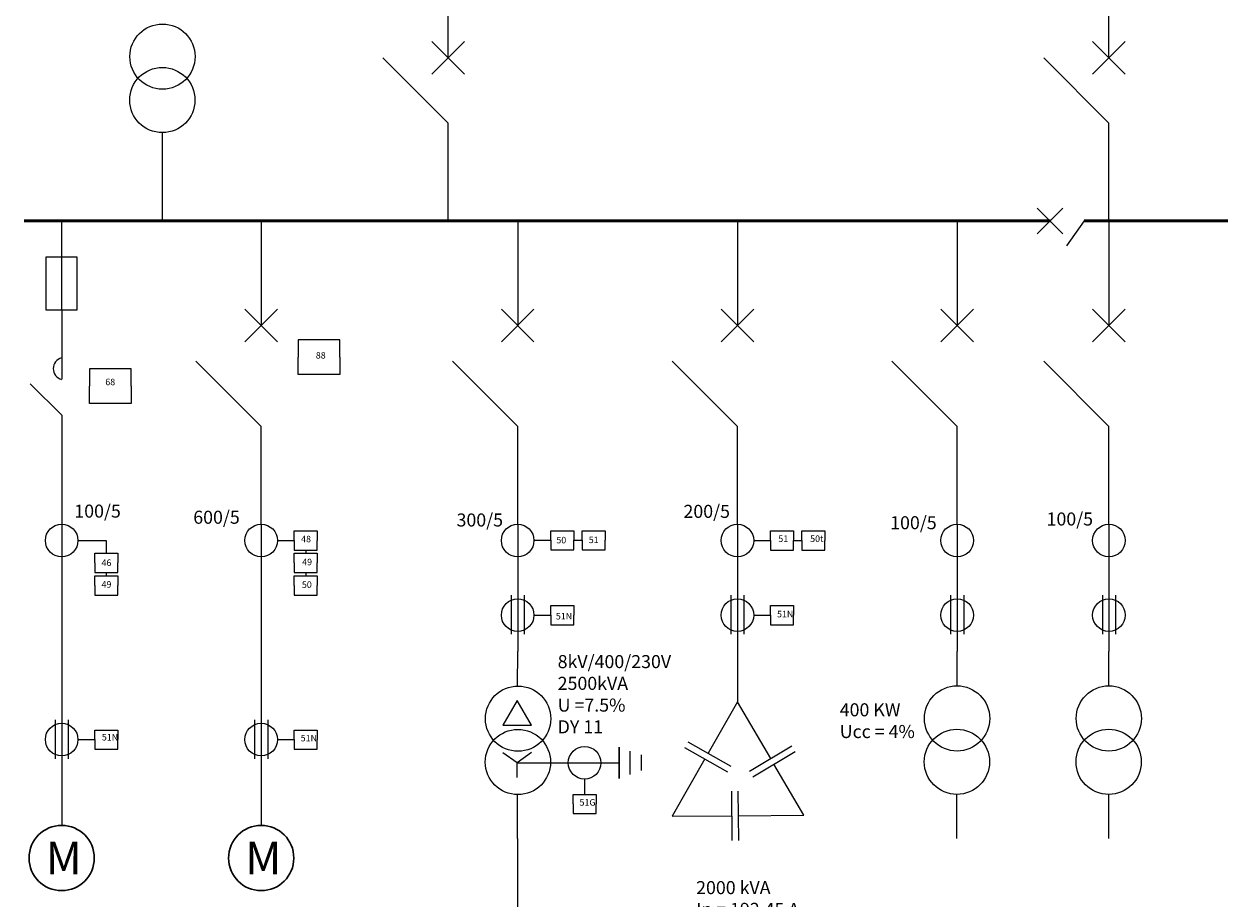
# Model space of a CAD drawing. Units: inches. Extents: x 77.1 to 95.7, y 45.4 to 81.6.
# Tile 2 of 3: x 77.2 to 95.6, y 58.2 to 71.6. Entities that reach past the tile are written whole.
import ezdxf

# ---------------------------------------------------------------- set-up
doc = ezdxf.new("R2010")
doc.units = ezdxf.units.IN
doc.header["$MEASUREMENT"] = 0
for name, color, linetype, lineweight in [('E-ANNO-TEXT', 7, 'Continuous', 18), ('E-POWR-BUSB', 7, 'Continuous', 50), ('E-POWR-CAPB', 3, 'Continuous', 25), ('E-POWR-CT', 4, 'Continuous', 18), ('E-POWR-EQPM', 3, 'Continuous', 30), ('E-POWR-FEED', 7, 'Continuous', 25), ('E-POWR-GRND', 3, 'Continuous', 18), ('E-POWR-SWCH', 1, 'Continuous', 25), ('E-POWR-XFMR', 4, 'Continuous', 25), ('E-PROT-RELY', 2, 'Continuous', 18), ('E-PROT-TEXT', 7, 'Continuous', 13), ('E-PROT-WIRE', 5, 'Continuous', 13)]:
    doc.layers.add(name, color=color, linetype=linetype, lineweight=lineweight)
doc.styles.get("Standard").update_dxf_attribs({"font": 'arial.ttf'})

# ---------------------------------------------------------------- blocks, each defined once
blk = doc.blocks.new('XFMR-TWO-WINDING')
for centre in [(0.502, 1.166), (0.5, 0.5)]:
    blk.add_circle(centre, 0.5)
blk = doc.blocks.new('CT-RESIDUAL')
for p, q in [((0.15, 0.598), (0.15, 0)), ((0.35, 0.598), (0.35, 0))]:
    blk.add_line(p, q)
blk.add_circle((0.25, 0.294), 0.25)
blk = doc.blocks.new('CT-SINGLE')
blk.add_circle((0.25, 0.25), 0.25)
blk = doc.blocks.new('MOTOR-AC')
blk.add_circle((0.5, 0.5), 0.5)
at = {"insert": (0.255, 0.75), "char_height": 0.5, "attachment_point": 1}
blk.add_mtext_dynamic_manual_height_columns('M', width=0.27964, gutter_width=1, heights=[0], dxfattribs=at)
blk = doc.blocks.new('EARTH-GROUND')
for p, q in [((0.174, 0.421), (0.174, 0.059)), ((0, 0.36), (0, 0.12))]:
    blk.add_line(p, q)
for points in [[(0.342, 0.24), (0.342, 0.24), (0.342, 0.48), (0.342, 0.48)], [(0.342, 0.24), (0.342, 0.24), (0.342, 0), (0.342, 0)]]:
    blk.add_lwpolyline(points, close=True)
blk = doc.blocks.new('CB-INCOMER-OPEN')
for p, q in [((0.75, 0.75), (1.25, 1.25)), ((0.75, 1.25), (1.25, 0.75)), ((1, 0), (0, 1))]:
    blk.add_line(p, q)
blk = doc.blocks.new('CB-FEEDER-OPEN')
for p, q in [((0.75, 1.299), (1.25, 1.799)), ((0.75, 1.799), (1.25, 1.299)), ((1, 0), (0, 1))]:
    blk.add_line(p, q)
blk = doc.blocks.new('RELAY-FUNCTION')
for p, q in [((0, 0.148), (0, 0.295)), ((0, 0.295), (0.353, 0.295)), ((0.353, 0.295), (0.353, 0.148)), ((0, 0.148), (0, 0)), ((0, 0), (0.353, 0)), ((0.353, 0), (0.353, 0.148))]:
    blk.add_line(p, q)
blk = doc.blocks.new('RELAY-FUNCTION-MED')
for p, q in [((0.638, 0.533), (0, 0.533)), ((0, 0.533), (0, 0.266)), ((0.638, 0.266), (0.638, 0.533)), ((0, 0), (0, 0.266)), ((0.638, 0.266), (0.638, 0)), ((0.638, 0), (0, 0))]:
    blk.add_line(p, q)

msp = doc.modelspace()

# ---------------------------------------------------------------- linework, layer by layer
at = {"layer": 'E-POWR-BUSB'}
for p, q in [((77.162, 68.605), (90.162, 68.605)), ((90.162, 68.605), (92.887, 68.605)), ((93.408, 68.605), (95.613, 68.605))]:
    msp.add_line(p, q, dxfattribs=at)
at = {"layer": 'E-POWR-CAPB'}
for p, q in [((87.95, 60.154), (87.291, 60.525)), ((87.999, 60.241), (87.34, 60.613)), ((88.279, 60.168), (88.93, 60.553)), ((88.33, 60.082), (88.981, 60.467)), ((88.002, 59.86), (88.01, 59.104)), ((88.102, 59.861), (88.11, 59.105))]:
    msp.add_line(p, q, dxfattribs=at)
for points in [[(88.605, 60.361), (88.094, 61.232), (87.645, 60.441)], [(87.595, 60.354), (87.096, 59.477), (88.006, 59.483)], [(88.106, 59.483), (89.115, 59.49), (88.655, 60.275)]]:
    msp.add_lwpolyline(points, dxfattribs=at)
at = {"layer": 'E-POWR-FEED'}
for p, q in [((83.662, 71.105), (83.662, 71.915)), ((93.789, 71.105), (93.789, 71.915)), ((79.284, 68.605), (79.281, 69.959)), ((83.662, 68.605), (83.662, 70.105)), ((93.789, 68.605), (93.789, 70.105)), ((77.738, 67.243), (77.738, 68.605)), ((80.796, 68.605), (80.796, 67.003)), ((84.727, 68.605), (84.727, 67.003)), ((88.095, 68.605), (88.095, 67.003)), ((91.463, 68.605), (91.463, 67.003)), ((93.789, 68.605), (93.789, 67.003)), ((77.738, 67.243), (77.738, 66.176)), ((77.738, 65.627), (77.738, 64.506)), ((80.796, 63.954), (80.796, 65.454)), ((84.727, 63.954), (84.727, 65.454)), ((88.095, 63.954), (88.095, 65.454)), ((91.463, 63.954), (91.463, 65.454)), ((93.789, 63.954), (93.789, 65.454)), ((77.738, 64.506), (77.738, 63.954)), ((77.738, 63.954), (77.738, 62.81)), ((80.796, 63.954), (80.796, 62.81)), ((84.727, 63.954), (84.727, 62.81)), ((88.095, 63.954), (88.095, 62.81)), ((91.463, 63.954), (91.463, 62.81)), ((93.789, 63.954), (93.789, 62.81)), ((77.738, 62.81), (77.738, 60.901)), ((80.796, 62.81), (80.796, 60.901)), ((84.727, 62.81), (84.727, 62.002)), ((88.095, 62.81), (88.095, 62.002)), ((91.463, 62.81), (91.463, 62.002)), ((93.789, 62.81), (93.789, 62.002)), ((84.725, 61.476), (84.727, 62.002)), ((88.095, 62.002), (88.095, 61.225)), ((91.461, 61.476), (91.463, 62.002)), ((93.787, 61.476), (93.789, 62.002)), ((77.738, 60.901), (77.738, 60.093)), ((80.796, 60.901), (80.796, 60.093)), ((77.738, 60.093), (77.738, 59.335)), ((80.796, 60.093), (80.796, 59.335)), ((84.724, 59.133), (84.723, 59.81)), ((91.46, 59.133), (91.459, 59.81)), ((93.786, 59.133), (93.785, 59.81)), ((84.724, 59.133), (84.724, 56.856))]:
    msp.add_line(p, q, dxfattribs=at)
at = {"layer": 'E-POWR-GRND'}
msp.add_line((84.719, 60.295), (86.281, 60.295), dxfattribs=at)
at = {"layer": 'E-POWR-SWCH'}
for p, q in [((92.691, 68.408), (93.084, 68.801)), ((92.691, 68.801), (93.084, 68.408)), ((93.408, 68.605), (93.14, 68.223)), ((77.976, 68.052), (77.496, 68.052)), ((77.496, 68.052), (77.496, 67.243)), ((77.976, 67.243), (77.976, 68.052)), ((77.496, 67.243), (77.738, 67.243)), ((77.738, 67.243), (77.976, 67.243)), ((77.738, 65.627), (77.257, 66.107))]:
    msp.add_line(p, q, dxfattribs=at)
msp.add_arc((77.779, 66.34), 0.17, 104.3094, 255.6906, dxfattribs=at)
at = {"layer": 'E-POWR-XFMR'}
msp.add_line((84.721, 60.072), (84.719, 60.295), dxfattribs=at)
msp.add_lwpolyline([(84.721, 61.251), (84.502, 60.871), (84.94, 60.871)], close=True, dxfattribs=at)
msp.add_lwpolyline([(84.937, 60.454), (84.719, 60.295), (84.498, 60.45)], dxfattribs=at)
for centre in [(84.733, 60.972), (84.731, 60.307)]:
    msp.add_circle(centre, 0.5, dxfattribs=at)
at = {"layer": 'E-PROT-WIRE'}
for p, q in [((77.988, 63.704), (78.244, 63.704)), ((78.244, 63.704), (78.42, 63.704)), ((78.42, 63.704), (78.42, 63.557)), ((81.046, 63.704), (81.302, 63.704)), ((84.977, 63.708), (85.234, 63.708)), ((85.586, 63.708), (85.715, 63.708)), ((88.345, 63.704), (88.601, 63.704)), ((88.954, 63.704), (89.082, 63.704)), ((78.42, 63.557), (78.42, 63.508)), ((81.479, 63.557), (81.479, 63.508)), ((78.42, 63.213), (78.42, 63.161)), ((81.479, 63.213), (81.479, 63.161)), ((84.977, 62.56), (85.233, 62.56)), ((88.345, 62.56), (88.601, 62.56)), ((77.988, 60.651), (78.244, 60.651)), ((81.046, 60.651), (81.302, 60.651)), ((85.753, 60.045), (85.753, 59.812))]:
    msp.add_line(p, q, dxfattribs=at)

# ---------------------------------------------------------------- block references
at = {"layer": 'E-POWR-CT'}
for name, p in [('CT-SINGLE', (77.488, 63.454)), ('CT-SINGLE', (80.546, 63.454)), ('CT-SINGLE', (84.477, 63.454)), ('CT-SINGLE', (87.845, 63.454)), ('CT-SINGLE', (91.213, 63.454)), ('CT-SINGLE', (93.539, 63.454)), ('CT-RESIDUAL', (84.477, 62.266)), ('CT-RESIDUAL', (87.845, 62.266)), ('CT-RESIDUAL', (91.213, 62.266)), ('CT-RESIDUAL', (93.539, 62.266)), ('CT-RESIDUAL', (77.488, 60.357)), ('CT-RESIDUAL', (80.546, 60.357)), ('CT-SINGLE', (85.503, 60.045))]:
    msp.add_blockref(name, p, dxfattribs=at)
at = {"layer": 'E-POWR-EQPM'}
for p in [(77.238, 58.335), (80.296, 58.335)]:
    msp.add_blockref('MOTOR-AC', p, dxfattribs=at)
at = {"layer": 'E-POWR-GRND', "rotation": 180}
msp.add_blockref('EARTH-GROUND', (86.623, 60.535), dxfattribs=at)
at = {"layer": 'E-POWR-SWCH'}
for name, p in [('CB-INCOMER-OPEN', (82.662, 70.105)), ('CB-INCOMER-OPEN', (92.789, 70.105)), ('CB-FEEDER-OPEN', (79.796, 65.454)), ('CB-FEEDER-OPEN', (83.727, 65.454)), ('CB-FEEDER-OPEN', (87.095, 65.454)), ('CB-FEEDER-OPEN', (90.463, 65.454)), ('CB-FEEDER-OPEN', (92.789, 65.454))]:
    msp.add_blockref(name, p, dxfattribs=at)
at = {"layer": 'E-POWR-XFMR'}
for p in [(78.781, 69.959), (90.959, 59.81), (93.285, 59.81)]:
    msp.add_blockref('XFMR-TWO-WINDING', p, dxfattribs=at)
at = {"layer": 'E-PROT-RELY'}
for name, p in [('RELAY-FUNCTION-MED', (81.365, 66.25)), ('RELAY-FUNCTION-MED', (78.167, 65.804)), ('RELAY-FUNCTION', (81.302, 63.556)), ('RELAY-FUNCTION', (85.234, 63.56)), ('RELAY-FUNCTION', (85.714, 63.56)), ('RELAY-FUNCTION', (88.601, 63.556)), ('RELAY-FUNCTION', (89.082, 63.556)), ('RELAY-FUNCTION', (78.244, 63.213)), ('RELAY-FUNCTION', (81.302, 63.213)), ('RELAY-FUNCTION', (78.244, 62.866)), ('RELAY-FUNCTION', (81.302, 62.866)), ('RELAY-FUNCTION', (85.233, 62.412)), ('RELAY-FUNCTION', (88.601, 62.412)), ('RELAY-FUNCTION', (78.244, 60.503)), ('RELAY-FUNCTION', (81.302, 60.503)), ('RELAY-FUNCTION', (85.576, 59.516))]:
    msp.add_blockref(name, p, dxfattribs=at)

# ---------------------------------------------------------------- texts
at = {"layer": 'E-ANNO-TEXT', "char_height": 0.2, "attachment_point": 1}
for s, width, insert in [('100/5', 0.93095, (77.932, 64.255)), ('200/5', 0.93095, (87.268, 64.251)), ('600/5', 0.93095, (79.755, 64.161)), ('300/5', 0.93095, (83.79, 64.119)), ('100/5', 0.93095, (90.436, 64.077)), ('100/5', 0.93095, (92.833, 64.134)), ('\\A1;{\\H1x;8}kV/400/230V\\P2500kVA\\PU =7.5% \\PDY 11', 2.97281, (85.34, 61.947)), ('400 KW\\PUcc = 4%', 2.97281, (89.663, 61.208)), ('2000 kVA\\PIn = 192.45 A', 2.97281, (87.462, 58.481))]:
    msp.add_mtext_dynamic_manual_height_columns(s, width=width, gutter_width=1, heights=[0], dxfattribs=dict(at, insert=insert))
at = {"layer": 'E-PROT-TEXT', "char_height": 0.1, "attachment_point": 1}
for s, insert in [('88', (81.633, 66.595)), ('68', (78.407, 66.186)), ('48', (81.408, 63.777)), ('50', (85.32, 63.76)), ('51', (85.816, 63.764)), ('51', (88.722, 63.782)), ('50t', (89.21, 63.782)), ('46', (78.349, 63.413)), ('49', (81.424, 63.425)), ('49', (78.349, 63.081)), ('50', (81.42, 63.077)), ('51N', (85.312, 62.593)), ('51N', (88.702, 62.626)), ('51N', (78.354, 60.737)), ('51N', (81.401, 60.724)), ('51G', (85.675, 59.738))]:
    msp.add_mtext_dynamic_manual_height_columns(s, width=0.27964, gutter_width=1, heights=[0], dxfattribs=dict(at, insert=insert))

doc.saveas('drawing.dxf')
